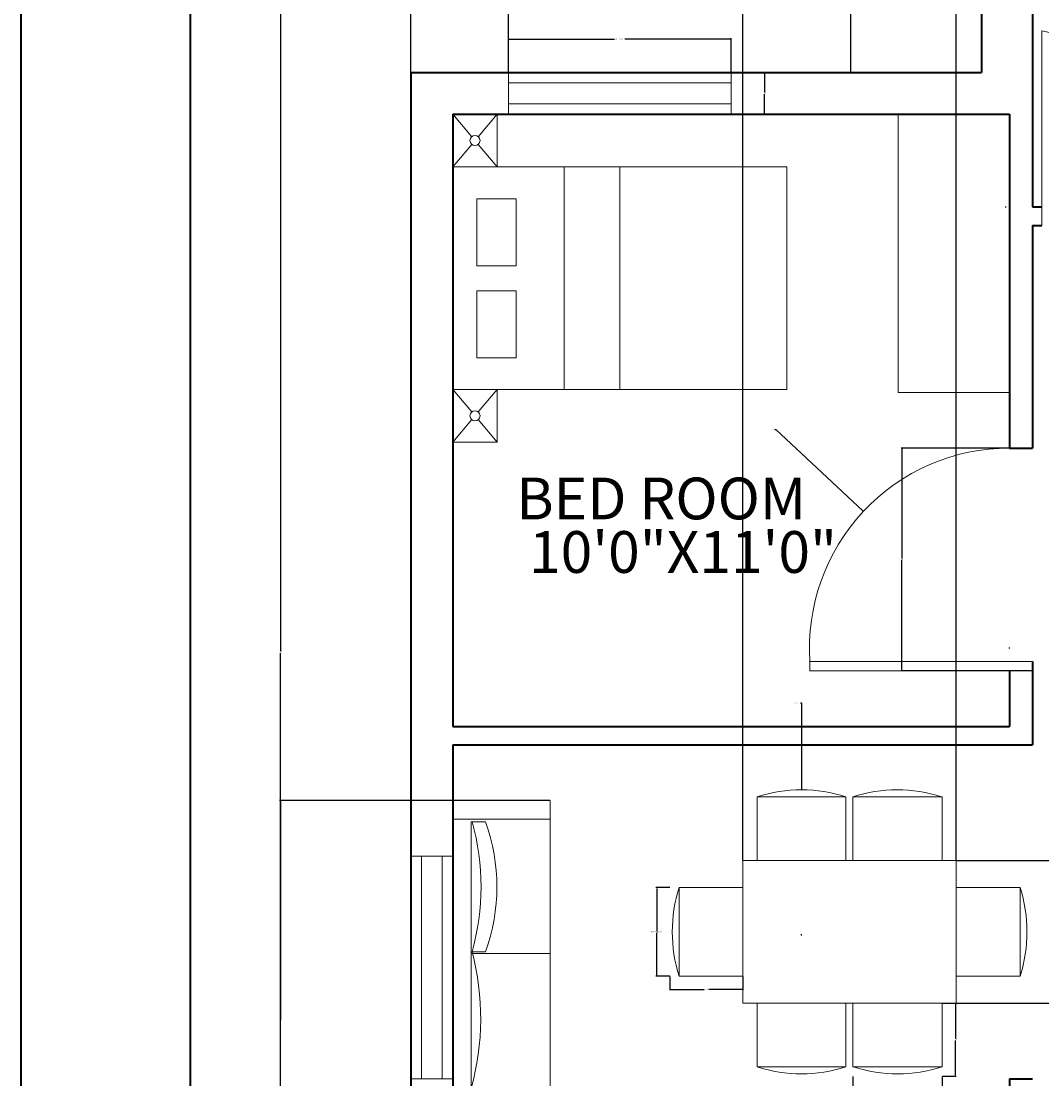
# Model space of a CAD drawing. Units: inches. Extents: x 1762 to 3150, y 1680 to 2382.
# Tile 2 of 6: x 1762 to 1983, y 1904 to 2132. Entities that reach past the tile are written whole.
import ezdxf

# ---------------------------------------------------------------- set-up
doc = ezdxf.new("R2010")
doc.units = ezdxf.units.IN
for name, color, linetype, lineweight in [('A-ANNO-DIMS', 2, 'Continuous', 18), ('A-ANNO-TTLB', 7, 'Continuous', 35), ('A-AREA-IDEN', 7, 'Continuous', 18), ('A-DOOR', 3, 'Continuous', 18), ('A-GLAZ', 4, 'Continuous', 18), ('A-WALL', 7, 'Continuous', 35)]:
    doc.layers.add(name, color=color, linetype=linetype, lineweight=lineweight)
doc.layers.add('A-FLOR-CASE', color=242, linetype='Continuous', lineweight=18, true_color=0xcd2027)
doc.layers.add('A-FURN', color=51, linetype='Continuous', lineweight=18, true_color=0xf7f281)
doc.styles.get("Standard").update_dxf_attribs({"font": 'arial.ttf'})
doc.dimstyles.get("Standard").update_dxf_attribs({"dimtxt": 0.18, "dimasz": 0.18, "dimexe": 0.18, "dimexo": 0.0625, "dimgap": 0.09, "dimtad": 0, "dimtih": 1, "dimtoh": 1, "dimdec": 4, "dimzin": 0, "dimdsep": 46, "dimtxsty": 'Standard', "dimcen": 0.09, "dimadec": 0, "dimazin": 0, "dimtfac": 1, "dimtdec": 4, "dimtofl": 0, "dimtmove": 0, "dimatfit": 3, "dimfxl": 1, "dimtolj": 1, "dimtzin": 0, "dimarcsym": 0})

# ---------------------------------------------------------------- blocks, each defined once
blk = doc.blocks.new('WINDOW-48IN')
for p, q in [((0, 48), (9, 48)), ((2.25, 48), (2.25, 0)), ((6.75, 48), (6.75, 0)), ((0, 0), (9, 0))]:
    blk.add_line(p, q)
blk = doc.blocks.new('BED-48X72IN')
for p, q in [((0, 72), (48, 72)), ((0, 72), (0, 0)), ((48, 72), (48, 0)), ((0, 36), (48, 36)), ((0, 24), (48, 24))]:
    blk.add_line(p, q)
for points in [[(6.88, 13.68), (21.36, 13.68), (21.36, 5.23), (6.88, 5.23)], [(26.73, 13.68), (41.21, 13.68), (41.21, 5.23), (26.73, 5.23)]]:
    blk.add_lwpolyline(points, close=True)
blk = doc.blocks.new('NIGHTSTAND')
for p, q in [((0, 9.61), (4.85, 5.5)), ((11.36, 9.61), (6.51, 5.5)), ((4.85, 4.1), (0, 0)), ((6.51, 4.1), (11.36, 0))]:
    blk.add_line(p, q)
blk.add_lwpolyline([(0, 9.61), (11.36, 9.61), (11.36, 0), (0, 0)], close=True)
blk.add_circle((5.68, 4.8), 1.08)
blk = doc.blocks.new('CHAIR-DINING')
for p, q in [((0, 0), (0, 13.75)), ((0, 13.75), (19.1, 13.75)), ((19.1, 0), (19.1, 13.75))]:
    blk.add_line(p, q)
blk.add_arc((9.55, -15.98), 31.23, 72.1947, 107.8053)
blk = doc.blocks.new('CHAIR-DINING-WIDE')
for p, q in [((0, 0), (0, 13.75)), ((0, 13.75), (19.24, 13.75)), ((19.24, 0), (19.24, 13.75))]:
    blk.add_line(p, q)
blk.add_arc((9.55, -15.98), 31.23, 72.1947, 107.8053)
blk = doc.blocks.new('WARDROBE-24X60IN')
for p, q in [((0, 60), (24, 60)), ((24, 60), (24, 0)), ((24, 0), (0, 0))]:
    blk.add_line(p, q)
blk = doc.blocks.new('*D18')
at = {"layer": 'A-ANNO-DIMS', "color": 0, "lineweight": -2, "transparency": 16777216}
for p, q in [((1867.54, 2121.05), (1867.54, 2128.37)), ((1867.72, 2128.19), (1890.42, 2128.19)), ((1915.36, 2128.19), (1892.66, 2128.19)), ((1915.54, 2121.05), (1915.54, 2128.37))]:
    blk.add_line(p, q, dxfattribs=at)
at = {"layer": 'A-ANNO-DIMS', "color": 0, "transparency": 16777216}
for points in [[(1867.72, 2128.22), (1867.72, 2128.16), (1867.54, 2128.19)], [(1915.36, 2128.22), (1915.36, 2128.16), (1915.54, 2128.19)]]:
    blk.add_solid(points, dxfattribs=at)
at = {"layer": 'Defpoints', "color": 0, "transparency": 16777216}
for p in [(1867.54, 2128.19), (1867.54, 2120.99), (1915.54, 2120.99)]:
    blk.add_point(p, dxfattribs=at)
at = {"layer": 'A-ANNO-DIMS', "color": 0, "transparency": 16777216, "insert": (1891.54, 2128.19), "char_height": 0.18, "attachment_point": 5}
blk.add_mtext('\\A1;WINDOW 48 TYP.', dxfattribs=at)
blk = doc.blocks.new('*D19')
at = {"layer": 'A-ANNO-DIMS', "color": 0, "lineweight": -2, "transparency": 16777216}
for p, q in [((1915.6, 2120.99), (1922.92, 2120.99)), ((1922.74, 2120.81), (1922.74, 2116.67)), ((1922.74, 2112.17), (1922.74, 2116.31)), ((1915.6, 2111.99), (1922.92, 2111.99))]:
    blk.add_line(p, q, dxfattribs=at)
at = {"layer": 'A-ANNO-DIMS', "color": 0, "transparency": 16777216}
for points in [[(1922.71, 2120.81), (1922.77, 2120.81), (1922.74, 2120.99)], [(1922.71, 2112.17), (1922.77, 2112.17), (1922.74, 2111.99)]]:
    blk.add_solid(points, dxfattribs=at)
at = {"layer": 'Defpoints', "color": 0, "transparency": 16777216}
for p in [(1915.54, 2120.99), (1922.74, 2120.99), (1915.54, 2111.99)]:
    blk.add_point(p, dxfattribs=at)
at = {"layer": 'A-ANNO-DIMS', "color": 0, "transparency": 16777216, "insert": (1922.74, 2116.49), "char_height": 0.18, "attachment_point": 5}
blk.add_mtext('\\A1;9 TYP.', dxfattribs=at)
blk = doc.blocks.new('*D20')
at = {"layer": 'A-ANNO-DIMS', "color": 0, "lineweight": -2, "transparency": 16777216}
for p, q in [((1902.31, 1945.23), (1899.33, 1945.23)), ((1899.51, 1945.05), (1899.51, 1935.87)), ((1899.51, 1926.32), (1899.51, 1935.5)), ((1902.31, 1926.14), (1899.33, 1926.14))]:
    blk.add_line(p, q, dxfattribs=at)
at = {"layer": 'A-ANNO-DIMS', "color": 0, "transparency": 16777216}
for points in [[(1899.48, 1945.05), (1899.54, 1945.05), (1899.51, 1945.23)], [(1899.48, 1926.32), (1899.54, 1926.32), (1899.51, 1926.14)]]:
    blk.add_solid(points, dxfattribs=at)
at = {"layer": 'Defpoints', "color": 0, "transparency": 16777216}
for p in [(1899.51, 1945.23), (1902.37, 1945.23), (1902.37, 1926.14)]:
    blk.add_point(p, dxfattribs=at)
at = {"layer": 'A-ANNO-DIMS', "color": 0, "transparency": 16777216, "insert": (1899.51, 1935.68), "char_height": 0.18, "attachment_point": 5}
blk.add_mtext('\\A1;DINING CHAIR 19 TYP.', dxfattribs=at)
blk = doc.blocks.new('*D21')
at = {"layer": 'A-ANNO-DIMS', "color": 0, "lineweight": -2, "transparency": 16777216}
for p, q in [((1902.37, 1926.07), (1902.37, 1923.09)), ((1918.11, 1926.07), (1918.11, 1923.09)), ((1902.55, 1923.27), (1909.72, 1923.27)), ((1917.93, 1923.27), (1910.76, 1923.27))]:
    blk.add_line(p, q, dxfattribs=at)
at = {"layer": 'A-ANNO-DIMS', "color": 0, "transparency": 16777216}
for points in [[(1902.55, 1923.3), (1902.55, 1923.24), (1902.37, 1923.27)], [(1917.93, 1923.3), (1917.93, 1923.24), (1918.11, 1923.27)]]:
    blk.add_solid(points, dxfattribs=at)
at = {"layer": 'Defpoints', "color": 0, "transparency": 16777216}
for p in [(1902.37, 1926.14), (1918.11, 1926.14), (1902.37, 1923.27)]:
    blk.add_point(p, dxfattribs=at)
at = {"layer": 'A-ANNO-DIMS', "color": 0, "transparency": 16777216, "insert": (1910.24, 1923.27), "char_height": 0.18, "attachment_point": 5}
blk.add_mtext('\\A1;16 TYP.', dxfattribs=at)
blk = doc.blocks.new('*D22')
at = {"layer": 'A-ANNO-DIMS', "color": 0, "lineweight": -2, "transparency": 16777216}
for p, q in [((1941.79, 1904.51), (1941.79, 1901.5)), ((1961.03, 1904.51), (1961.03, 1901.5)), ((1941.97, 1901.68), (1950.09, 1901.68)), ((1960.85, 1901.68), (1952.73, 1901.68))]:
    blk.add_line(p, q, dxfattribs=at)
at = {"layer": 'A-ANNO-DIMS', "color": 0, "transparency": 16777216}
for points in [[(1941.97, 1901.71), (1941.97, 1901.65), (1941.79, 1901.68)], [(1960.85, 1901.71), (1960.85, 1901.65), (1961.03, 1901.68)]]:
    blk.add_solid(points, dxfattribs=at)
at = {"layer": 'Defpoints', "color": 0, "transparency": 16777216}
for p in [(1941.79, 1904.57), (1961.03, 1904.57), (1941.79, 1901.68)]:
    blk.add_point(p, dxfattribs=at)
at = {"layer": 'A-ANNO-DIMS', "color": 0, "transparency": 16777216, "insert": (1951.41, 1901.68), "char_height": 0.18, "attachment_point": 5}
blk.add_mtext('\\A1;WIDE CHAIR 19 TYP.', dxfattribs=at)
blk = doc.blocks.new('*D23')
at = {"layer": 'A-ANNO-DIMS', "color": 0, "lineweight": -2, "transparency": 16777216}
for p, q in [((1961.09, 1920.31), (1964.1, 1920.31)), ((1963.92, 1920.13), (1963.92, 1912.62)), ((1963.92, 1904.75), (1963.92, 1912.26)), ((1961.09, 1904.57), (1964.1, 1904.57))]:
    blk.add_line(p, q, dxfattribs=at)
at = {"layer": 'A-ANNO-DIMS', "color": 0, "transparency": 16777216}
for points in [[(1963.89, 1920.13), (1963.95, 1920.13), (1963.92, 1920.31)], [(1963.89, 1904.75), (1963.95, 1904.75), (1963.92, 1904.57)]]:
    blk.add_solid(points, dxfattribs=at)
at = {"layer": 'Defpoints', "color": 0, "transparency": 16777216}
for p in [(1961.03, 1920.31), (1961.03, 1904.57), (1963.92, 1904.57)]:
    blk.add_point(p, dxfattribs=at)
at = {"layer": 'A-ANNO-DIMS', "color": 0, "transparency": 16777216, "insert": (1963.92, 1912.44), "char_height": 0.18, "attachment_point": 5}
blk.add_mtext('\\A1;16 TYP.', dxfattribs=at)
blk = doc.blocks.new('*D32')
at = {"layer": 'A-ANNO-DIMS', "color": 0, "lineweight": -2, "transparency": 16777216}
for p, q in [((1846.54, 2121.05), (1846.54, 2325.32)), ((1846.72, 2325.14), (2005.25, 2325.14)), ((2164.36, 2325.14), (2005.83, 2325.14)), ((2164.54, 2092.05), (2164.54, 2325.32))]:
    blk.add_line(p, q, dxfattribs=at)
at = {"layer": 'A-ANNO-DIMS', "color": 0, "transparency": 16777216}
for points in [[(1846.72, 2325.17), (1846.72, 2325.11), (1846.54, 2325.14)], [(2164.36, 2325.17), (2164.36, 2325.11), (2164.54, 2325.14)]]:
    blk.add_solid(points, dxfattribs=at)
at = {"layer": 'Defpoints', "color": 0, "transparency": 16777216}
for p in [(2164.54, 2325.14), (1846.54, 2120.99), (2164.54, 2091.99)]:
    blk.add_point(p, dxfattribs=at)
at = {"layer": 'A-ANNO-DIMS', "color": 0, "transparency": 16777216, "insert": (2005.54, 2325.14), "char_height": 0.18, "attachment_point": 5}
blk.add_mtext('\\A1;318', dxfattribs=at)
blk = doc.blocks.new('*D33')
at = {"layer": 'A-ANNO-DIMS', "color": 0, "lineweight": -2, "transparency": 16777216}
for p, q in [((1969.475966, 2232.98945), (1818.208466, 2232.98945)), ((1818.388466, 2232.80945), (1818.388466, 1996.16945)), ((1818.388466, 1759.16945), (1818.388466, 1995.80945)), ((1846.475966, 1758.98945), (1818.208466, 1758.98945))]:
    blk.add_line(p, q, dxfattribs=at)
at = {"layer": 'A-ANNO-DIMS', "color": 0, "transparency": 16777216}
for points in [[(1818.358466, 2232.80945), (1818.418466, 2232.80945), (1818.388466, 2232.98945)], [(1818.358466, 1759.16945), (1818.418466, 1759.16945), (1818.388466, 1758.98945)]]:
    blk.add_solid(points, dxfattribs=at)
at = {"layer": 'Defpoints', "color": 0, "transparency": 16777216}
for p in [(1818.388466, 2232.98945), (1969.538466, 2232.98945), (1846.538466, 1758.98945)]:
    blk.add_point(p, dxfattribs=at)
at = {"layer": 'A-ANNO-DIMS', "color": 0, "transparency": 16777216, "insert": (1818.388466, 1995.98945), "char_height": 0.18, "attachment_point": 5}
blk.add_mtext('\\A1;474', dxfattribs=at)
blk = doc.blocks.new('*D44')
at = {"layer": 'A-ANNO-DIMS', "color": 0, "lineweight": -2, "transparency": 16777216}
for p, q in [((1969.48, 2232.99), (1941.21, 2232.99)), ((1941.39, 2232.81), (1941.39, 2177.17)), ((1941.39, 2121.17), (1941.39, 2176.81)), ((1969.48, 2120.99), (1941.21, 2120.99))]:
    blk.add_line(p, q, dxfattribs=at)
at = {"layer": 'A-ANNO-DIMS', "color": 0, "transparency": 16777216}
for points in [[(1941.36, 2232.81), (1941.42, 2232.81), (1941.39, 2232.99)], [(1941.36, 2121.17), (1941.42, 2121.17), (1941.39, 2120.99)]]:
    blk.add_solid(points, dxfattribs=at)
at = {"layer": 'Defpoints', "color": 0, "transparency": 16777216}
for p in [(1941.39, 2232.99), (1969.54, 2232.99), (1969.54, 2120.99)]:
    blk.add_point(p, dxfattribs=at)
at = {"layer": 'A-ANNO-DIMS', "color": 0, "transparency": 16777216, "insert": (1941.39, 2176.99), "char_height": 0.18, "attachment_point": 5}
blk.add_mtext('\\A1;112', dxfattribs=at)
blk = doc.blocks.new('*D45')
at = {"layer": 'A-ANNO-DIMS', "color": 0, "lineweight": -2, "transparency": 16777216}
for p, q in [((1846.54, 2121.05), (1846.54, 2149.32)), ((1846.72, 2149.14), (1856.84, 2149.14)), ((1867.36, 2149.14), (1857.24, 2149.14)), ((1867.54, 2121.05), (1867.54, 2149.32))]:
    blk.add_line(p, q, dxfattribs=at)
at = {"layer": 'A-ANNO-DIMS', "color": 0, "transparency": 16777216}
for points in [[(1846.72, 2149.17), (1846.72, 2149.11), (1846.54, 2149.14)], [(1867.36, 2149.17), (1867.36, 2149.11), (1867.54, 2149.14)]]:
    blk.add_solid(points, dxfattribs=at)
at = {"layer": 'Defpoints', "color": 0, "transparency": 16777216}
for p in [(1867.54, 2149.14), (1846.54, 2120.99), (1867.54, 2120.99)]:
    blk.add_point(p, dxfattribs=at)
at = {"layer": 'A-ANNO-DIMS', "color": 0, "transparency": 16777216, "insert": (1857.04, 2149.14), "char_height": 0.18, "attachment_point": 5}
blk.add_mtext('\\A1;21', dxfattribs=at)
blk = doc.blocks.new('*D50')
at = {"layer": 'A-ANNO-DIMS', "color": 0, "lineweight": -2, "transparency": 16777216}
for p, q in [((1980.48, 2039.99), (1952.21, 2039.99)), ((1952.39, 2039.81), (1952.39, 2016.17)), ((1952.39, 1992.17), (1952.39, 2015.81)), ((1980.48, 1991.99), (1952.21, 1991.99))]:
    blk.add_line(p, q, dxfattribs=at)
at = {"layer": 'A-ANNO-DIMS', "color": 0, "transparency": 16777216}
for points in [[(1952.36, 2039.81), (1952.42, 2039.81), (1952.39, 2039.99)], [(1952.36, 1992.17), (1952.42, 1992.17), (1952.39, 1991.99)]]:
    blk.add_solid(points, dxfattribs=at)
at = {"layer": 'Defpoints', "color": 0, "transparency": 16777216}
for p in [(1952.39, 2039.99), (1980.54, 2039.99), (1980.54, 1991.99)]:
    blk.add_point(p, dxfattribs=at)
at = {"layer": 'A-ANNO-DIMS', "color": 0, "transparency": 16777216, "insert": (1952.39, 2015.99), "char_height": 0.18, "attachment_point": 5}
blk.add_mtext('\\A1;48', dxfattribs=at)
blk = doc.blocks.new('*D57')
at = {"layer": 'A-ANNO-DIMS', "color": 0, "lineweight": -2, "transparency": 16777216}
for p, q in [((1918.11, 1951.12), (1918.11, 2325.32)), ((1918.29, 2325.14), (1940.7, 2325.14)), ((1963.91, 2325.14), (1941.5, 2325.14)), ((1964.09, 1951.12), (1964.09, 2325.32))]:
    blk.add_line(p, q, dxfattribs=at)
at = {"layer": 'A-ANNO-DIMS', "color": 0, "transparency": 16777216}
for points in [[(1918.29, 2325.17), (1918.29, 2325.11), (1918.11, 2325.14)], [(1963.91, 2325.17), (1963.91, 2325.11), (1964.09, 2325.14)]]:
    blk.add_solid(points, dxfattribs=at)
at = {"layer": 'Defpoints', "color": 0, "transparency": 16777216}
for p in [(1964.09, 2325.14), (1918.11, 1951.05), (1964.09, 1951.05)]:
    blk.add_point(p, dxfattribs=at)
at = {"layer": 'A-ANNO-DIMS', "color": 0, "transparency": 16777216, "insert": (1941.1, 2325.14), "char_height": 0.18, "attachment_point": 5}
blk.add_mtext('\\A1;45.97', dxfattribs=at)
blk = doc.blocks.new('*D58')
at = {"layer": 'A-ANNO-DIMS', "color": 0, "lineweight": -2, "transparency": 16777216}
for p, q in [((1964.15, 1951.05), (2192.87, 1951.05)), ((2192.69, 1950.87), (2192.69, 1935.87)), ((2192.69, 1920.49), (2192.69, 1935.5)), ((1964.15, 1920.31), (2192.87, 1920.31))]:
    blk.add_line(p, q, dxfattribs=at)
at = {"layer": 'A-ANNO-DIMS', "color": 0, "transparency": 16777216}
for points in [[(2192.66, 1950.87), (2192.72, 1950.87), (2192.69, 1951.05)], [(2192.66, 1920.49), (2192.72, 1920.49), (2192.69, 1920.31)]]:
    blk.add_solid(points, dxfattribs=at)
at = {"layer": 'Defpoints', "color": 0, "transparency": 16777216}
for p in [(1964.09, 1951.05), (1964.09, 1920.31), (2192.69, 1920.31)]:
    blk.add_point(p, dxfattribs=at)
at = {"layer": 'A-ANNO-DIMS', "color": 0, "transparency": 16777216, "insert": (2192.69, 1935.68), "char_height": 0.18, "attachment_point": 5}
blk.add_mtext('\\A1;30.74', dxfattribs=at)
blk = doc.blocks.new('*D60')
at = {"layer": 'A-ANNO-DIMS', "color": 0, "lineweight": -2, "transparency": 16777216}
for p, q in [((1876.48, 1963.99), (1818.21, 1963.99)), ((1818.39, 1963.81), (1818.39, 1916.67)), ((1818.39, 1869.17), (1818.39, 1916.31)), ((1876.48, 1868.99), (1818.21, 1868.99))]:
    blk.add_line(p, q, dxfattribs=at)
at = {"layer": 'A-ANNO-DIMS', "color": 0, "transparency": 16777216}
for points in [[(1818.36, 1963.81), (1818.42, 1963.81), (1818.39, 1963.99)], [(1818.36, 1869.17), (1818.42, 1869.17), (1818.39, 1868.99)]]:
    blk.add_solid(points, dxfattribs=at)
at = {"layer": 'Defpoints', "color": 0, "transparency": 16777216}
for p in [(1818.39, 1963.99), (1876.54, 1963.99), (1876.54, 1868.99)]:
    blk.add_point(p, dxfattribs=at)
at = {"layer": 'A-ANNO-DIMS', "color": 0, "transparency": 16777216, "insert": (1818.39, 1916.49), "char_height": 0.18, "attachment_point": 5}
blk.add_mtext('\\A1;95', dxfattribs=at)
blk = doc.blocks.new('*D95')
at = {"layer": 'A-ANNO-DIMS', "color": 0, "lineweight": -2, "transparency": 16777216}
for p, q in [((1930.54, 1985.03), (1930.72, 1985.03)), ((1930.72, 1985.03), (1930.72, 1966.48)), ((1930.63, 1935.07), (1930.81, 1935.07)), ((1930.72, 1934.98), (1930.72, 1935.16))]:
    blk.add_line(p, q, dxfattribs=at)
at = {"layer": 'A-ANNO-DIMS', "color": 0, "transparency": 16777216}
blk.add_solid([(1930.75, 1966.48), (1930.69, 1966.48), (1930.72, 1966.3)], dxfattribs=at)
at = {"layer": 'Defpoints', "color": 0, "transparency": 16777216}
for p in [(1930.72, 1966.3), (1930.72, 1935.07)]:
    blk.add_point(p, dxfattribs=at)
at = {"layer": 'A-ANNO-DIMS', "color": 0, "transparency": 16777216, "insert": (1929.79, 1985.03), "char_height": 0.18, "attachment_point": 5}
blk.add_mtext('\\A1;6X R31.225', dxfattribs=at)
blk = doc.blocks.new('*D96')
at = {"layer": 'A-ANNO-DIMS', "color": 0, "lineweight": -2, "transparency": 16777216}
for p, q in [((1924.98, 2043.98), (1925.16, 2043.98)), ((1925.16, 2043.98), (1943.92, 2026.44)), ((1975.45, 1996.89), (1975.63, 1996.89)), ((1975.54, 1996.8), (1975.54, 1996.98))]:
    blk.add_line(p, q, dxfattribs=at)
at = {"layer": 'A-ANNO-DIMS', "color": 0, "transparency": 16777216}
blk.add_solid([(1943.94, 2026.47), (1943.9, 2026.42), (1944.05, 2026.32)], dxfattribs=at)
at = {"layer": 'Defpoints', "color": 0, "transparency": 16777216}
for p in [(1944.05, 2026.32), (1975.54, 1996.89)]:
    blk.add_point(p, dxfattribs=at)
at = {"layer": 'A-ANNO-DIMS', "color": 0, "transparency": 16777216, "insert": (1924.59, 2043.98), "char_height": 0.18, "attachment_point": 5}
blk.add_mtext('\\A1;R43.1', dxfattribs=at)
blk = doc.blocks.new('*D99')
at = {"layer": 'A-ANNO-DIMS', "color": 0, "lineweight": -2, "transparency": 16777216}
for p, q in [((2022.84, 2131.22), (2004.94, 2116.62)), ((2023.02, 2131.22), (2022.84, 2131.22)), ((1974.66, 2091.99), (1974.84, 2091.99)), ((1974.75, 2091.9), (1974.75, 2092.08))]:
    blk.add_line(p, q, dxfattribs=at)
at = {"layer": 'A-ANNO-DIMS', "color": 0, "transparency": 16777216}
blk.add_solid([(2004.93, 2116.65), (2004.96, 2116.6), (2004.81, 2116.51)], dxfattribs=at)
at = {"layer": 'Defpoints', "color": 0, "transparency": 16777216}
for p in [(2004.81, 2116.51), (1974.75, 2091.99)]:
    blk.add_point(p, dxfattribs=at)
at = {"layer": 'A-ANNO-DIMS', "color": 0, "transparency": 16777216, "insert": (2023.5, 2131.22), "char_height": 0.18, "attachment_point": 5}
blk.add_mtext('\\A1;R38.79', dxfattribs=at)

msp = doc.modelspace()

# ---------------------------------------------------------------- linework, layer by layer
at = {"layer": 'A-ANNO-TTLB'}
for points in [[(1762.4998, 2382.3025), (3150.3176, 2382.3025), (3150.3176, 1679.5742), (1762.4998, 1679.5742)], [(1799.0337, 2359.5805), (3111.4319, 2359.5805), (3111.4319, 1709.6712), (1799.0337, 1709.6712)]]:
    msp.add_lwpolyline(points, close=True, dxfattribs=at)
at = {"layer": 'A-DOOR'}
for p, q in [((1982.5385, 2129.9895), (1982.5385, 2087.9895)), ((1932.5385, 1993.9895), (1932.5385, 1991.9895)), ((1932.5385, 1993.9895), (1980.5385, 1993.9895)), ((1932.5385, 1991.9895), (1980.5385, 1991.9895))]:
    msp.add_line(p, q, dxfattribs=at)
for centre, radius, start, end in [((1974.7481, 2091.9894), 38.7903, 360, 78.414407), ((1975.5385, 1996.8916), 43.0978, 90, 183.861175)]:
    msp.add_arc(centre, radius, start, end, dxfattribs=at)
at = {"layer": 'A-FURN'}
for p, q in [((1855.5385, 1963.9895), (1876.5385, 1963.9895)), ((1876.5385, 1963.9895), (1876.5385, 1868.9895)), ((1855.5385, 1959.9895), (1876.5385, 1959.9895)), ((1859.5385, 1959.9895), (1862.6768, 1959.9895)), ((1859.5385, 1959.375), (1859.5385, 1872.9895)), ((1859.5385, 1959.375), (1862.6201, 1959.375)), ((1859.5385, 1948.868), (1859.5385, 1872.9895)), ((1859.5385, 1930.9895), (1876.5385, 1930.9895)), ((1859.7077, 1931.409), (1862.6201, 1931.409))]:
    msp.add_line(p, q, dxfattribs=at)
msp.add_lwpolyline([(1918.1134, 1951.0543), (1964.0853, 1951.0543), (1964.0853, 1920.3134), (1918.1134, 1920.3134)], close=True, dxfattribs=at)
for centre, radius, start, end in [((1810.0656, 1945.4058), 51.5776, 344.253959, 15.714157), ((1823.5839, 1945.392), 41.4651, 340.292171, 19.707829), ((1804.8495, 1917.0143), 56.7154, 344.638036, 14.70288)]:
    msp.add_arc(centre, radius, start, end, dxfattribs=at)
at = {"layer": 'A-WALL'}
for p, q in [((1969.5385, 2232.9895), (1969.5385, 2120.9895)), ((1980.5385, 2223.9895), (1980.5385, 2091.9894)), ((1846.5385, 2120.9895), (1969.5385, 2120.9895)), ((1846.5385, 2120.9895), (1846.5385, 1758.9895)), ((1855.5385, 2111.9895), (1975.5385, 2111.9895)), ((1855.5385, 2111.9895), (1855.5385, 1979.9895)), ((1975.5385, 2111.9895), (1975.5385, 2039.9895)), ((1975.5385, 2111.9895), (1975.5385, 2039.9895)), ((1980.5385, 2091.9894), (1982.5385, 2091.9894)), ((1980.5385, 2087.9895), (1982.5385, 2087.9895)), ((1980.5385, 2087.9895), (1980.5385, 2039.9895)), ((1975.5385, 2039.9895), (1980.5385, 2039.9895)), ((1980.5385, 1993.9895), (1980.5385, 1975.9895)), ((1975.5385, 1991.9895), (1975.5385, 1979.9895)), ((1975.5385, 1991.9895), (1975.5385, 1979.9895)), ((1855.5385, 1979.9895), (1975.5385, 1979.9895)), ((1855.5385, 1975.9895), (1980.5385, 1975.9895)), ((1855.5385, 1975.9895), (1855.5385, 1767.9895)), ((1975.5385, 1903.9895), (1975.5385, 1767.9895)), ((1975.5385, 1903.9895), (1980.5385, 1903.9895))]:
    msp.add_line(p, q, dxfattribs=at)

# ---------------------------------------------------------------- block references
at = {"layer": 'A-FLOR-CASE', "rotation": 180}
msp.add_blockref('WARDROBE-24X60IN', (1975.5389, 2111.9899), dxfattribs=at)
at = {"layer": 'A-FURN'}
for name, p, rotation in [('NIGHTSTAND', (1855.538, 2111.9898), 269.9999999999998), ('BED-48X72IN', (1855.538, 2100.6328), 270.0000000000011), ('NIGHTSTAND', (1855.538, 2052.6326), 269.9999999999966), ('CHAIR-DINING', (1918.1137, 1926.1357), 89.99999999998995), ('CHAIR-DINING', (1964.085, 1945.2319), 270.0000000000078), ('CHAIR-DINING', (1940.2652, 1920.3136), 180), ('CHAIR-DINING-WIDE', (1961.0299, 1920.3136), 180)]:
    msp.add_blockref(name, p, dxfattribs=dict(at, rotation=rotation))
for name, p in [('CHAIR-DINING', (1921.169, 1951.054)), ('CHAIR-DINING-WIDE', (1941.793, 1951.054))]:
    msp.add_blockref(name, p, dxfattribs=at)
at = {"layer": 'A-GLAZ', "rotation": 89.99999999999905}
msp.add_blockref('WINDOW-48IN', (1915.5389, 2111.989), dxfattribs=at)
at = {"layer": 'A-GLAZ'}
msp.add_blockref('WINDOW-48IN', (1846.538, 1903.989), dxfattribs=at)

# ---------------------------------------------------------------- texts
at = {"layer": 'A-AREA-IDEN'}
for s, p in [('BED ROOM', (1869.2436, 2024.6273)), (' 10\'0"X11\'0"', (1869.2436, 2013.0882))]:
    msp.add_text(s, height=9, dxfattribs=at).set_placement(p)

# ---------------------------------------------------------------- dimensions: what is measured, and where the dimension line sits
at = {"layer": 'A-ANNO-DIMS'}
for base, p1, p2, override, picture, middle in [((2164.5385, 2325.1356), (1846.5385, 2120.9895), (2164.5385, 2091.9894), {"dimdec": 0, "dimlfac": 1, "dimrnd": 0, "dimzin": 0, "dimdsep": 46, "dimlunit": 2}, '*D32', (2005.5385, 2325.1356)), ((1964.0853, 2325.1356), (1918.1134, 1951.0543), (1964.0853, 1951.0543), {"dimdec": 2, "dimlfac": 1, "dimrnd": 0, "dimzin": 0, "dimdsep": 46, "dimlunit": 2}, '*D57', (1941.0994, 2325.1356)), ((1867.5385, 2149.1395), (1846.5385, 2120.9895), (1867.5385, 2120.9895), {"dimdec": 0, "dimlfac": 1, "dimrnd": 0, "dimzin": 0, "dimdsep": 46, "dimlunit": 2}, '*D45', (1857.0385, 2149.1395))]:
    dim = msp.add_linear_dim(base=base, p1=p1, p2=p2, dimstyle='Standard', override=override, dxfattribs=at)
    dim.commit()
    dim.dimension.update_dxf_attribs({"geometry": picture, "text_midpoint": middle})
for base, p1, p2, override, picture, middle in [((1818.3885, 2232.9895), (1846.5385, 1758.9895), (1969.5385, 2232.9895), {"dimdec": 0, "dimlfac": 1, "dimrnd": 0, "dimzin": 0, "dimdsep": 46, "dimlunit": 2}, '*D33', (1818.3885, 1995.9895)), ((1941.3885, 2232.9895), (1969.5385, 2120.9895), (1969.5385, 2232.9895), {"dimdec": 0, "dimlfac": 1, "dimrnd": 0, "dimzin": 0, "dimdsep": 46, "dimlunit": 2}, '*D44', (1941.3885, 2176.9895)), ((1952.3885, 2039.9895), (1980.5385, 1991.9895), (1980.5385, 2039.9895), {"dimdec": 0, "dimlfac": 1, "dimrnd": 0, "dimzin": 0, "dimdsep": 46, "dimlunit": 2}, '*D50', (1952.3885, 2015.9895)), ((1818.3885, 1963.9895), (1876.5385, 1868.9895), (1876.5385, 1963.9895), {"dimdec": 0, "dimlfac": 1, "dimrnd": 0, "dimzin": 0, "dimdsep": 46, "dimlunit": 2}, '*D60', (1818.3885, 1916.4895)), ((2192.6885, 1920.3134), (1964.0853, 1951.0543), (1964.0853, 1920.3134), {"dimdec": 2, "dimlfac": 1, "dimrnd": 0, "dimzin": 0, "dimdsep": 46, "dimlunit": 2}, '*D58', (2192.6885, 1935.6838))]:
    dim = msp.add_linear_dim(base=base, p1=p1, p2=p2, angle=90, dimstyle='Standard', override=override, dxfattribs=at)
    dim.commit()
    dim.dimension.update_dxf_attribs({"geometry": picture, "text_midpoint": middle})
for center, mpoint, override, picture, middle in [((1974.7481, 2091.9894), (2004.8052, 2116.5101), {"dimdec": 2, "dimlfac": 1, "dimrnd": 0, "dimzin": 0, "dimdsep": 46, "dimlunit": 2}, '*D99', (2023.4994, 2131.2226)), ((1975.5385, 1996.8916), (1944.054, 2026.322), {"dimdec": 1, "dimlfac": 1, "dimrnd": 0, "dimzin": 0, "dimdsep": 46, "dimlunit": 2}, '*D96', (1924.5907, 2043.9803))]:
    dim = msp.add_radius_dim(center=center, mpoint=mpoint, dimstyle='Standard', override=override, dxfattribs=at)
    dim.commit()
    dim.dimension.update_dxf_attribs({"geometry": picture, "text_midpoint": middle, "dimtype": 164})
for base, p1, p2, angle, text, picture, middle in [((1867.5385, 2128.1895), (1915.5385, 2120.9895), (1867.5385, 2120.9895), 180, 'WINDOW <> TYP.', '*D18', (1891.5385, 2128.1895)), ((1922.7385, 2120.9895), (1915.5385, 2111.9895), (1915.5385, 2120.9895), 90, '<> TYP.', '*D19', (1922.7385, 2116.4895)), ((1899.5053, 1945.2321), (1902.3697, 1926.1356), (1902.3697, 1945.2321), 90, 'DINING CHAIR <> TYP.', '*D20', (1899.5053, 1935.6838)), ((1902.3697, 1923.2711), (1918.1134, 1926.1356), (1902.3697, 1926.1356), 180, '<> TYP.', '*D21', (1910.2416, 1923.2711)), ((1963.9154, 1904.5697), (1961.0299, 1920.3134), (1961.0299, 1904.5697), 270, '<> TYP.', '*D23', (1963.9154, 1912.4415)), ((1941.793, 1901.6842), (1961.0299, 1904.5697), (1941.793, 1904.5697), 180, 'WIDE CHAIR <> TYP.', '*D22', (1951.4115, 1901.6842))]:
    dim = msp.add_linear_dim(base=base, p1=p1, p2=p2, angle=angle, text=text, dimstyle='Standard', override={"dimdec": 0, "dimlfac": 1, "dimrnd": 0, "dimzin": 0, "dimdsep": 46, "dimlunit": 2}, dxfattribs=at)
    dim.commit()
    dim.dimension.update_dxf_attribs({"geometry": picture, "text_midpoint": middle})
dim = msp.add_radius_dim(center=(1930.7171, 1935.074), mpoint=(1930.717, 1966.2994), text='6X <>', dimstyle='Standard', override={"dimdec": 3, "dimlfac": 1, "dimrnd": 0, "dimzin": 0, "dimdsep": 46, "dimlunit": 2}, dxfattribs=at)
dim.commit()
dim.dimension.update_dxf_attribs({"geometry": '*D95', "text_midpoint": (1929.7926, 1985.0346), "dimtype": 164})

doc.saveas('drawing.dxf')
